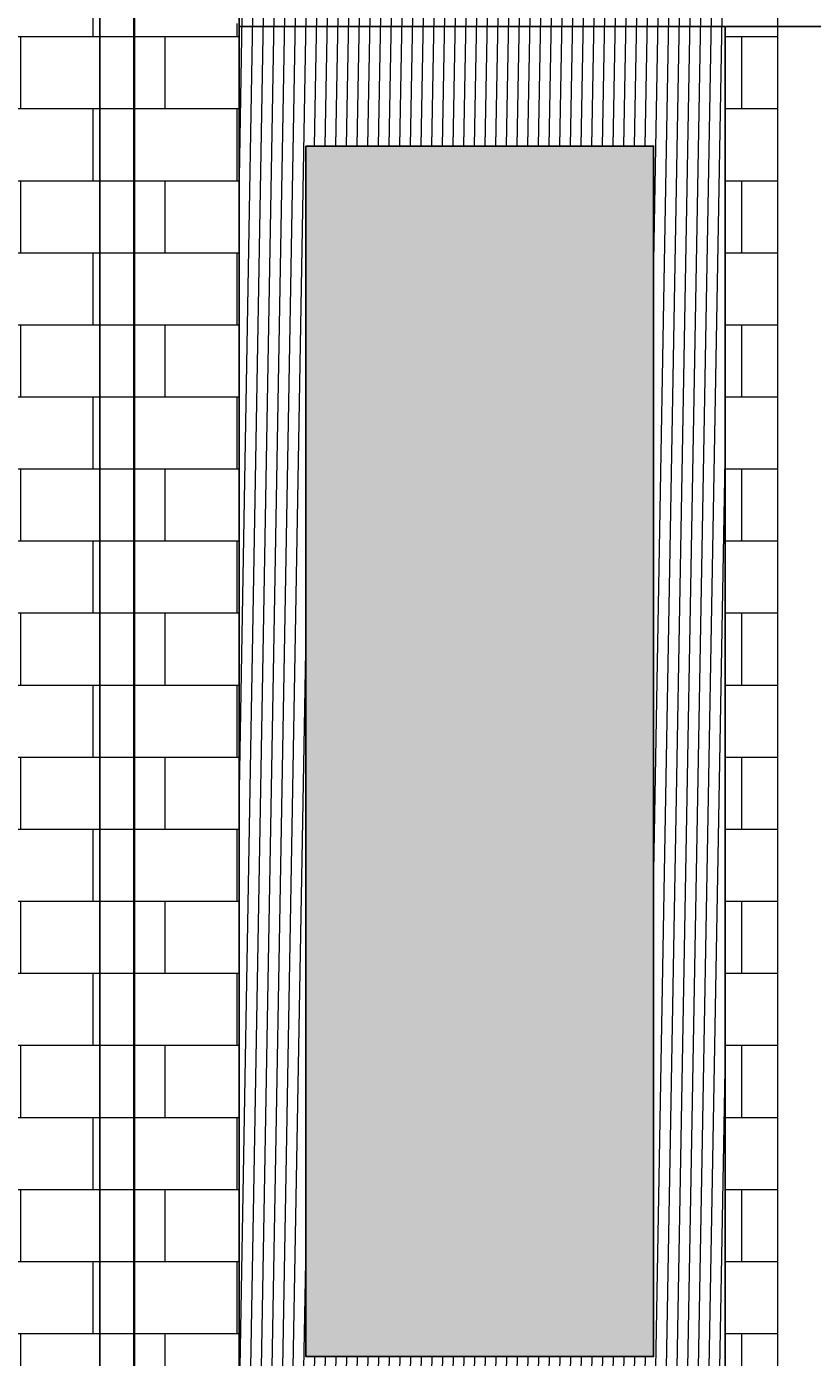
# Model space of a CAD drawing. Units: inches. Extents: x -26 to 776, y -22 to 650.
# Tile 15 of 62: x 222 to 288, y 34 to 145. Entities that reach past the tile are written whole.
import ezdxf

# ---------------------------------------------------------------- set-up
doc = ezdxf.new("R2010")
doc.units = ezdxf.units.IN
doc.header["$MEASUREMENT"] = 0
for name, color, linetype, lineweight in [('A-ANNO-DIMS', 2, 'Continuous', 18), ('A-DETL-PATT', 8, 'Continuous', 13), ('A-DOOR', 3, 'Continuous', 25), ('A-DOOR-PATT', 8, 'Continuous', 13), ('A-WALL', 7, 'Continuous', 35), ('A-WALL-PATT', 8, 'Continuous', 13), ('A-WALL-TRIM', 7, 'Continuous', 18)]:
    doc.layers.add(name, color=color, linetype=linetype, lineweight=lineweight)
doc.styles.get("Standard").update_dxf_attribs({"font": 'arial.ttf'})
doc.dimstyles.get("Standard").update_dxf_attribs({"dimtxt": 0.5625, "dimasz": 0.18, "dimexe": 0.18, "dimexo": 0.0625, "dimgap": 0.09, "dimtad": 0, "dimtih": 1, "dimtoh": 1, "dimdec": 4, "dimzin": 0, "dimdsep": 46, "dimlunit": 4, "dimtxsty": 'Standard', "dimcen": 0.09, "dimadec": 0, "dimazin": 0, "dimtfac": 1, "dimtdec": 4, "dimtofl": 0, "dimtmove": 0, "dimatfit": 3, "dimfxl": 1, "dimtolj": 1, "dimtzin": 0, "dimarcsym": 0})

# ---------------------------------------------------------------- blocks, each defined once
blk = doc.blocks.new('*D13')
at = {"layer": 'A-ANNO-DIMS', "color": 0, "lineweight": -2, "transparency": 16777216}
for p, q in [((738.75, 50.79), (738.75, -21.31)), ((11.11, 15.42), (11.11, -21.31)), ((11.29, -21.13), (373.89, -21.13)), ((738.57, -21.13), (375.97, -21.13))]:
    blk.add_line(p, q, dxfattribs=at)
at = {"layer": 'A-ANNO-DIMS', "color": 0, "transparency": 16777216}
for points in [[(11.29, -21.1), (11.29, -21.16), (11.11, -21.13)], [(738.57, -21.1), (738.57, -21.16), (738.75, -21.13)]]:
    blk.add_solid(points, dxfattribs=at)
at = {"layer": 'Defpoints', "color": 0, "transparency": 16777216}
for p in [(738.75, 50.85), (11.11, 15.48), (738.75, -21.13)]:
    blk.add_point(p, dxfattribs=at)
at = {"layer": 'A-ANNO-DIMS', "color": 0, "transparency": 16777216, "insert": (374.93, -21.13), "char_height": 0.562, "attachment_point": 5}
blk.add_mtext('\\A1;727.6', dxfattribs=at)
blk = doc.blocks.new('*D30')
at = {"layer": 'A-ANNO-DIMS', "color": 0, "lineweight": -2, "transparency": 16777216}
for p, q in [((280.68, 144.84), (775.34, 144.84)), ((775.16, 144.66), (775.16, 86.01)), ((775.16, 26.6), (775.16, 85.25)), ((280.68, 26.42), (775.34, 26.42))]:
    blk.add_line(p, q, dxfattribs=at)
at = {"layer": 'A-ANNO-DIMS', "color": 0, "transparency": 16777216}
for points in [[(775.13, 144.66), (775.19, 144.66), (775.16, 144.84)], [(775.13, 26.6), (775.19, 26.6), (775.16, 26.42)]]:
    blk.add_solid(points, dxfattribs=at)
at = {"layer": 'Defpoints', "color": 0, "transparency": 16777216}
for p in [(280.62, 144.84), (775.16, 144.84), (280.62, 26.42)]:
    blk.add_point(p, dxfattribs=at)
at = {"layer": 'A-ANNO-DIMS', "color": 0, "transparency": 16777216, "insert": (775.16, 85.63), "char_height": 0.562, "attachment_point": 5}
blk.add_mtext('\\A1;118.41', dxfattribs=at)
blk = doc.blocks.new('*D34')
at = {"layer": 'A-ANNO-DIMS', "color": 0, "lineweight": -2, "transparency": 16777216}
for p, q in [((228.57, 528.3), (228.57, -21.31)), ((357.3, 528.36), (357.3, -21.31)), ((228.75, -21.13), (291.71, -21.13)), ((357.12, -21.13), (294.17, -21.13))]:
    blk.add_line(p, q, dxfattribs=at)
at = {"layer": 'A-ANNO-DIMS', "color": 0, "transparency": 16777216}
for points in [[(228.75, -21.1), (228.75, -21.16), (228.57, -21.13)], [(357.12, -21.1), (357.12, -21.16), (357.3, -21.13)]]:
    blk.add_solid(points, dxfattribs=at)
at = {"layer": 'Defpoints', "color": 0, "transparency": 16777216}
for p in [(228.57, 528.36), (357.3, 528.42), (357.3, -21.13)]:
    blk.add_point(p, dxfattribs=at)
at = {"layer": 'A-ANNO-DIMS', "color": 0, "transparency": 16777216, "insert": (292.94, -21.13), "char_height": 0.562, "attachment_point": 5}
blk.add_mtext('\\A1;128.73', dxfattribs=at)
blk = doc.blocks.new('*D37')
at = {"layer": 'A-ANNO-DIMS', "color": 0, "lineweight": -2, "transparency": 16777216}
for p, q in [((231.36, 159.48), (-25.48, 159.48)), ((-25.3, 159.3), (-25.3, 87.85)), ((-25.3, 15.66), (-25.3, 87.11)), ((217.89, 15.48), (-25.48, 15.48))]:
    blk.add_line(p, q, dxfattribs=at)
at = {"layer": 'A-ANNO-DIMS', "color": 0, "transparency": 16777216}
for points in [[(-25.33, 159.3), (-25.27, 159.3), (-25.3, 159.48)], [(-25.33, 15.66), (-25.27, 15.66), (-25.3, 15.48)]]:
    blk.add_solid(points, dxfattribs=at)
at = {"layer": 'Defpoints', "color": 0, "transparency": 16777216}
for p in [(-25.3, 159.48), (231.42, 159.48), (217.95, 15.48)]:
    blk.add_point(p, dxfattribs=at)
at = {"layer": 'A-ANNO-DIMS', "color": 0, "transparency": 16777216, "insert": (-25.3, 87.48), "char_height": 0.562, "attachment_point": 5}
blk.add_mtext('\\A1;144', dxfattribs=at)
blk = doc.blocks.new('*D44')
at = {"layer": 'A-ANNO-DIMS', "color": 0, "lineweight": -2, "transparency": 16777216}
for p, q in [((231.42, 15.54), (231.42, 649.86)), ((231.6, 649.68), (234.98, 649.68)), ((239.99, 649.68), (236.61, 649.68)), ((240.17, 26.49), (240.17, 649.86))]:
    blk.add_line(p, q, dxfattribs=at)
at = {"layer": 'A-ANNO-DIMS', "color": 0, "transparency": 16777216}
for points in [[(231.6, 649.71), (231.6, 649.65), (231.42, 649.68)], [(239.99, 649.71), (239.99, 649.65), (240.17, 649.68)]]:
    blk.add_solid(points, dxfattribs=at)
at = {"layer": 'Defpoints', "color": 0, "transparency": 16777216}
for p in [(240.17, 649.68), (240.17, 26.42), (231.42, 15.48)]:
    blk.add_point(p, dxfattribs=at)
at = {"layer": 'A-ANNO-DIMS', "color": 0, "transparency": 16777216, "insert": (235.8, 649.68), "char_height": 0.562, "attachment_point": 5}
blk.add_mtext('\\A1;8.74', dxfattribs=at)

msp = doc.modelspace()

# ---------------------------------------------------------------- hatches: boundary and pattern name
at = {"layer": 'A-DETL-PATT'}
h = msp.add_hatch(dxfattribs=at)
h.set_pattern_fill('ANSI31', color=256, scale=7.1, angle=44)
h.paths.add_polyline_path([(231.4249, 197.3298), (216.1056, 197.3298), (216.1056, 159.4824), (231.4249, 159.4824)])
h.paths.add_polyline_path([(236.4647, 197.3298), (231.4249, 197.3298), (231.4249, 159.4824), (276.1134, 159.4824), (276.1134, 171.4173), (236.4647, 171.4173)])
h.paths.add_polyline_path([(259.7413, 197.3298), (236.4647, 197.3298), (236.4647, 171.4173), (259.7413, 171.4173)], flags=17)
h.paths.add_polyline_path([(276.1134, 197.3298), (261.7413, 197.3298), (261.7413, 171.4173), (276.1134, 171.4173)], flags=17)
h.paths.add_polyline_path([(217.9529, 147.0781), (22.8891, 147.0781), (22.8891, 138.3844), (217.9529, 138.3844)])
h.paths.add_polyline_path([(285.0179, 152.3087), (285.0179, 159.4824), (231.4249, 159.4824), (240.1654, 144.8359), (280.6173, 144.8359)])
h.paths.add_polyline_path([(280.6173, 144.8359), (240.1654, 144.8359), (240.1654, 26.4239), (280.6173, 26.4239)])
h.paths.add_polyline_path([(274.6644, 134.8811), (274.6644, 34.0885), (245.7207, 34.0885), (245.7207, 134.8811)], flags=16)
h.paths.add_polyline_path([(285.0179, 303.3046), (236.4647, 303.3046), (236.4647, 294.4171), (285.0179, 294.4171)])
h.paths.add_polyline_path([(285.0179, 446.0063), (236.4647, 446.0063), (236.4647, 437.1188), (285.0179, 437.1188)])
at = {"layer": 'A-DOOR-PATT'}
h = msp.add_hatch(color=256, dxfattribs=at)
h.dxf.hatch_style = 1
h.paths.add_polyline_path([(217.9529, 138.3844), (22.8891, 138.3844), (22.8891, 124.9232), (217.9529, 124.9232)])
h.paths.add_polyline_path([(274.6644, 134.8811), (245.7207, 134.8811), (245.7207, 34.0885), (274.6644, 34.0885)])
at = {"layer": 'A-WALL-PATT'}
h = msp.add_hatch(dxfattribs=at)
h.set_pattern_fill('AR-B816', color=256, scale=0.75)
h.paths.add_polyline_path([(82.134, 209.6413), (11.1074, 209.6413), (11.1074, 159.4824), (82.134, 159.4824)])
h.paths.add_polyline_path([(231.4249, 209.6413), (209.091, 209.6413), (209.091, 159.4824), (214.1056, 159.4824), (214.1056, 199.3298), (231.4249, 199.3298)])
h.paths.add_polyline_path([(231.4249, 159.4824), (11.1074, 159.4824), (11.1074, 22.5014), (22.8891, 22.5014), (22.8891, 147.0781), (217.9529, 147.0781), (217.9529, 20.7937), (231.4249, 20.7937)])
h.paths.add_polyline_path([(285.0179, 152.3087), (280.6173, 144.8359), (280.6173, 26.4239), (240.1654, 26.4239), (240.1654, 144.8359), (231.4249, 159.4824), (231.4249, 20.7937), (285.0179, 20.7937)])

# ---------------------------------------------------------------- linework, layer by layer
at = {"layer": 'A-DOOR'}
for points in [[(240.1654, 144.8359), (280.6173, 144.8359), (280.6173, 26.4239), (240.1654, 26.4239)], [(245.7207, 134.8811), (274.6644, 134.8811), (274.6644, 34.0885), (245.7207, 34.0885)]]:
    msp.add_lwpolyline(points, close=True, dxfattribs=at)
at = {"layer": 'A-WALL'}
msp.add_line((231.4249, 159.4824), (231.4249, 15.4824), dxfattribs=at)
at = {"layer": 'A-WALL-TRIM'}
msp.add_line((285.0179, 15.4824), (285.0179, 249.6598), dxfattribs=at)

# ---------------------------------------------------------------- dimensions: what is measured, and where the dimension line sits
at = {"layer": 'A-ANNO-DIMS'}
for base, p1, p2, override, picture, middle in [((240.1654, 649.6763), (231.4249, 15.4824), (240.1654, 26.4239), {"dimdec": 2, "dimlfac": 1, "dimrnd": 0, "dimzin": 0, "dimdsep": 46, "dimlunit": 2}, '*D44', (235.7952, 649.6763)), ((357.3034, -21.1349), (228.5733, 528.3585), (357.3034, 528.4233), {"dimdec": 2, "dimlfac": 1, "dimrnd": 0, "dimzin": 0, "dimdsep": 46, "dimlunit": 2}, '*D34', (292.9384, -21.1349)), ((738.7503, -21.1349), (11.1074, 15.4824), (738.7503, 50.8482), {"dimdec": 1, "dimlfac": 1, "dimrnd": 0, "dimzin": 0, "dimdsep": 46, "dimlunit": 2}, '*D13', (374.9289, -21.1349))]:
    dim = msp.add_linear_dim(base=base, p1=p1, p2=p2, dimstyle='Standard', override=override, dxfattribs=at)
    dim.commit()
    dim.dimension.update_dxf_attribs({"geometry": picture, "text_midpoint": middle})
for base, p1, p2, override, picture, middle in [((-25.2976, 159.4824), (217.9529, 15.4824), (231.4249, 159.4824), {"dimdec": 0, "dimlfac": 1, "dimrnd": 0, "dimzin": 0, "dimdsep": 46, "dimlunit": 2}, '*D37', (-25.2976, 87.4824)), ((775.1553, 144.8359), (280.6173, 26.4239), (280.6173, 144.8359), {"dimdec": 2, "dimlfac": 1, "dimrnd": 0, "dimzin": 0, "dimdsep": 46, "dimlunit": 2}, '*D30', (775.1553, 85.6299))]:
    dim = msp.add_linear_dim(base=base, p1=p1, p2=p2, angle=90, dimstyle='Standard', override=override, dxfattribs=at)
    dim.commit()
    dim.dimension.update_dxf_attribs({"geometry": picture, "text_midpoint": middle})

doc.saveas('drawing.dxf')
